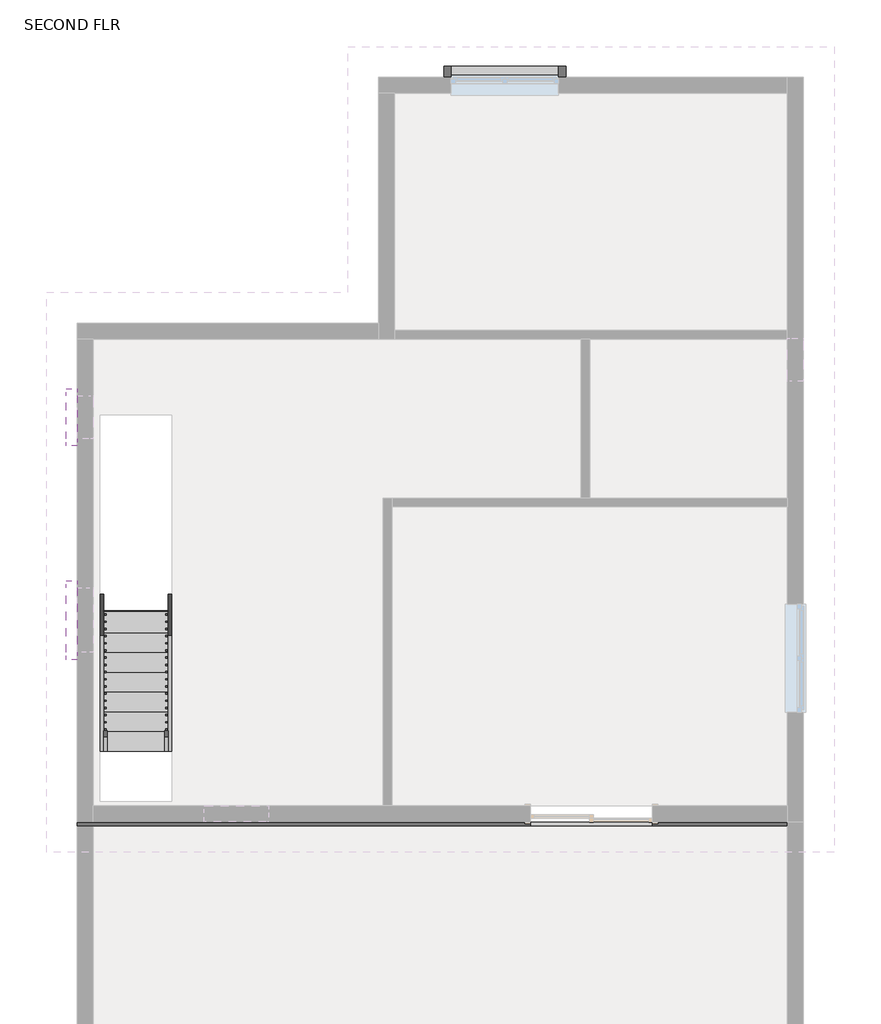
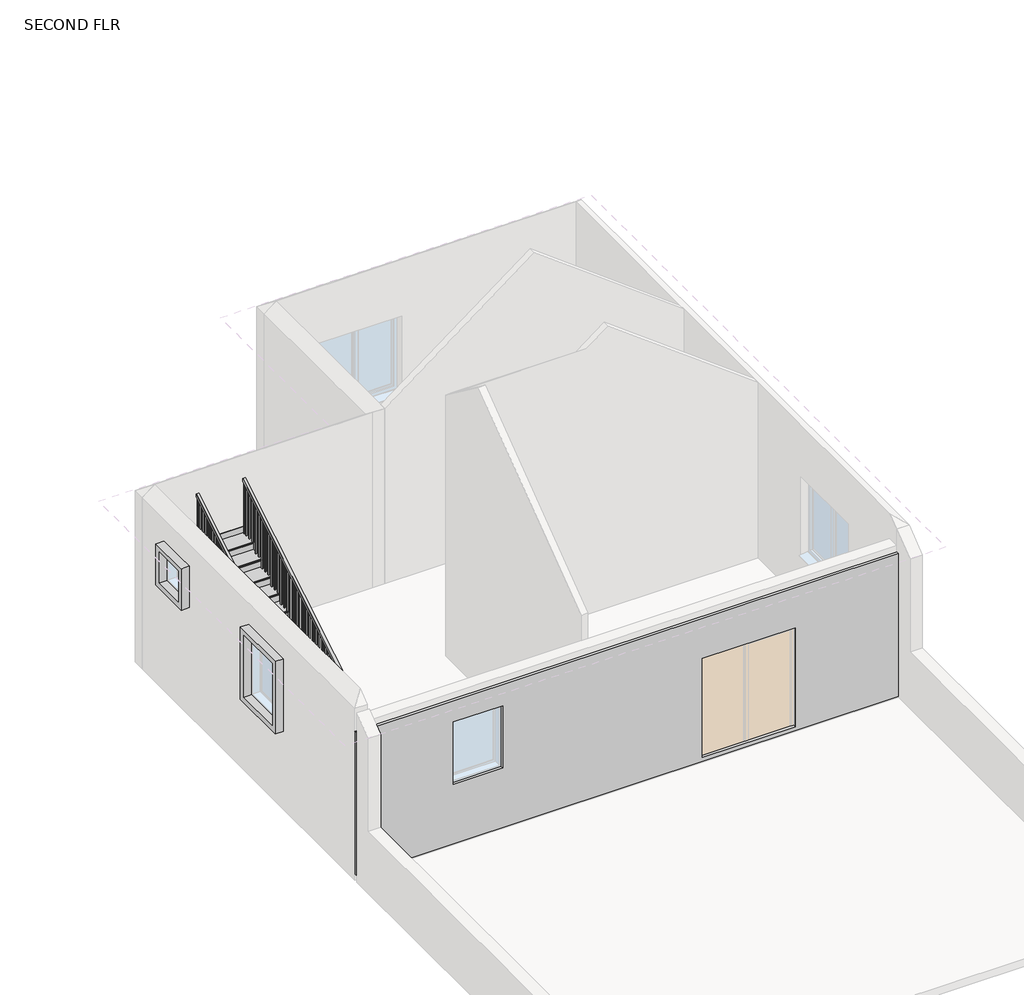
# One storey, part 2 of 2: 4 proxies, 2 members, 2 railings, 1 stair flight.
"""IFC4 building model written with IfcOpenShell, lengths in millimetres."""

from ifc_helpers import new_model, si_unit, frame, origin, place, context, project, spatial, polyline, outline, extrude, transform, mapped, element, save
from components import generic_models_10_generic_models_10_8dbd4941, generic_models_18_generic_models_18_bc45088a, generic_models_5_generic_models_5_2da6e60e, generic_models_9_generic_models_9_c35f1afa, stair_flight_ac41b8a3

model = new_model("IFC4")

# Units and contexts
model_context = context("Model", 3, world=origin())
ifc_project = project(units=[si_unit("LENGTHUNIT", "METRE", prefix="MILLI")], contexts=[model_context])

# Site, building, storey
site = spatial("IfcSite", under=ifc_project)
building = spatial("IfcBuilding", under=site)
storey = spatial("IfcBuildingStorey", under=building, Name="SECOND FLR", Elevation=6400.8)

# Proxies
placement = place(None, origin())
generic_models_10_generic_models_10_shape = generic_models_10_generic_models_10_8dbd4941(model_context)
element("IfcBuildingElementProxy", 1, Name="Generic Models 10 : Generic Models 10", ObjectType="Generic Models 10 : Generic Models 10", at=placement, inside=storey, context=model_context, shape_type="MappedRepresentation", body=[
    mapped(generic_models_10_generic_models_10_shape, transform((0.0, 0.0, 0.0), x_axis=(1.0, 0.0, 0.0), y_axis=(0.0, 1.0, 0.0), z_axis=(0.0, 0.0, 1.0))),
])
generic_models_18_generic_models_18_shape = generic_models_18_generic_models_18_bc45088a(model_context)
element("IfcBuildingElementProxy", 2, Name="Generic Models 18 : Generic Models 18", ObjectType="Generic Models 18 : Generic Models 18", at=placement, inside=storey, context=model_context, shape_type="MappedRepresentation", body=[
    mapped(generic_models_18_generic_models_18_shape, transform((0.0, 0.0, 0.0), x_axis=(1.0, 0.0, 0.0), y_axis=(0.0, 1.0, 0.0), z_axis=(0.0, 0.0, 1.0))),
])
generic_models_5_generic_models_5_shape = generic_models_5_generic_models_5_2da6e60e(model_context)
element("IfcBuildingElementProxy", 3, Name="Generic Models 5 : Generic Models 5", ObjectType="Generic Models 5 : Generic Models 5", at=placement, inside=storey, context=model_context, shape_type="MappedRepresentation", body=[
    mapped(generic_models_5_generic_models_5_shape, transform((0.0, 0.0, 0.0), x_axis=(1.0, 0.0, 0.0), y_axis=(0.0, 1.0, 0.0), z_axis=(0.0, 0.0, 1.0))),
])
generic_models_9_generic_models_9_shape = generic_models_9_generic_models_9_c35f1afa(model_context)
element("IfcBuildingElementProxy", 4, Name="Generic Models 9 : Generic Models 9", ObjectType="Generic Models 9 : Generic Models 9", at=placement, inside=storey, context=model_context, shape_type="MappedRepresentation", body=[
    mapped(generic_models_9_generic_models_9_shape, transform((0.0, 0.0, 0.0), x_axis=(1.0, 0.0, 0.0), y_axis=(0.0, 1.0, 0.0), z_axis=(0.0, 0.0, 1.0))),
])

# Members
element("IfcMember", 5, ObjectType="Stringer - 2\" Width", at=placement, inside=storey, context=model_context, shape_type="SweptSolid", body=[
    extrude(outline(polyline([(2731.9325341, 6400.8), (2731.9325341, 6612.914512), (7481.7325341, 9491.5811786), (7481.7325341, 9135.1724171), (2970.0180459, 6400.8), (2731.9325341, 6400.8)])), frame((-5772.3875748, 0.0, 0.0), z_axis=(1.0, 0.0, 0.0), x_axis=(0.0, 1.0, 0.0)), (0.0, 0.0, 1.0), 50.8),
])
element("IfcMember", 6, ObjectType="Stringer - 2\" Width", at=placement, inside=storey, context=model_context, shape_type="SweptSolid", body=[
    extrude(outline(polyline([(2731.9325341, 6400.8), (2731.9325341, 6612.914512), (7481.7325341, 9491.5811786), (7481.7325341, 9135.1724171), (2970.0180459, 6400.8), (2731.9325341, 6400.8)])), frame((-4807.1875748, 0.0, 0.0), z_axis=(1.0, 0.0, 0.0), x_axis=(0.0, 1.0, 0.0)), (0.0, 0.0, 1.0), 50.8),
])

# Railings
element("IfcRailing", 7, ObjectType="Handrail - Rectangular", at=placement, inside=storey, context=model_context, shape_type="SweptSolid", body=[
    extrude(outline(polyline([(2731.9325341, 7425.1318731), (2731.9325341, 7484.5333333), (7481.7325341, 10363.2), (7481.7325341, 10303.7985397), (2731.9325341, 7425.1318731)])), frame((-4857.9875748, 0.0, 0.0), z_axis=(1.0, 0.0, 0.0), x_axis=(0.0, 1.0, 0.0)), (0.0, 0.0, 1.0), 50.8),
    extrude(outline(polyline([(7396.0075341, 10251.8439943), (7415.0575341, 10263.3894488), (7415.0575341, 9279.4666667), (7396.0075341, 9279.4666667), (7396.0075341, 10251.8439943)])), frame((-4842.1125748, 0.0, 0.0), z_axis=(1.0, 0.0, 0.0), x_axis=(0.0, 1.0, 0.0)), (0.0, 0.0, 1.0), 19.05),
    extrude(outline(polyline([(7294.4075341, 10190.2682367), (7313.4575341, 10201.8136913), (7313.4575341, 9279.4666667), (7294.4075341, 9279.4666667), (7294.4075341, 10190.2682367)])), frame((-4842.1125748, 0.0, 0.0), z_axis=(1.0, 0.0, 0.0), x_axis=(0.0, 1.0, 0.0)), (0.0, 0.0, 1.0), 19.05),
    extrude(outline(polyline([(7192.8075341, 10128.6924791), (7211.8575341, 10140.2379337), (7211.8575341, 9279.4666667), (7192.8075341, 9279.4666667), (7192.8075341, 10128.6924791)])), frame((-4842.1125748, 0.0, 0.0), z_axis=(1.0, 0.0, 0.0), x_axis=(0.0, 1.0, 0.0)), (0.0, 0.0, 1.0), 19.05),
    extrude(outline(polyline([(7091.2075341, 10067.1167216), (7110.2575341, 10078.6621761), (7110.2575341, 9110.1333333), (7091.2075341, 9110.1333333), (7091.2075341, 10067.1167216)])), frame((-4842.1125748, 0.0, 0.0), z_axis=(1.0, 0.0, 0.0), x_axis=(0.0, 1.0, 0.0)), (0.0, 0.0, 1.0), 19.05),
    extrude(outline(polyline([(6989.6075341, 10005.540964), (7008.6575341, 10017.0864185), (7008.6575341, 9110.1333333), (6989.6075341, 9110.1333333), (6989.6075341, 10005.540964)])), frame((-4842.1125748, 0.0, 0.0), z_axis=(1.0, 0.0, 0.0), x_axis=(0.0, 1.0, 0.0)), (0.0, 0.0, 1.0), 19.05),
    extrude(outline(polyline([(6888.0075341, 9943.9652064), (6907.0575341, 9955.510661), (6907.0575341, 8940.8), (6888.0075341, 8940.8), (6888.0075341, 9943.9652064)])), frame((-4842.1125748, 0.0, 0.0), z_axis=(1.0, 0.0, 0.0), x_axis=(0.0, 1.0, 0.0)), (0.0, 0.0, 1.0), 19.05),
    extrude(outline(polyline([(6786.4075341, 9882.3894488), (6805.4575341, 9893.9349034), (6805.4575341, 8940.8), (6786.4075341, 8940.8), (6786.4075341, 9882.3894488)])), frame((-4842.1125748, 0.0, 0.0), z_axis=(1.0, 0.0, 0.0), x_axis=(0.0, 1.0, 0.0)), (0.0, 0.0, 1.0), 19.05),
    extrude(outline(polyline([(6684.8075341, 9820.8136913), (6703.8575341, 9832.3591458), (6703.8575341, 8940.8), (6684.8075341, 8940.8), (6684.8075341, 9820.8136913)])), frame((-4842.1125748, 0.0, 0.0), z_axis=(1.0, 0.0, 0.0), x_axis=(0.0, 1.0, 0.0)), (0.0, 0.0, 1.0), 19.05),
    extrude(outline(polyline([(6583.2075341, 9759.2379337), (6602.2575341, 9770.7833882), (6602.2575341, 8771.4666667), (6583.2075341, 8771.4666667), (6583.2075341, 9759.2379337)])), frame((-4842.1125748, 0.0, 0.0), z_axis=(1.0, 0.0, 0.0), x_axis=(0.0, 1.0, 0.0)), (0.0, 0.0, 1.0), 19.05),
    extrude(outline(polyline([(6481.6075341, 9697.6621761), (6500.6575341, 9709.2076307), (6500.6575341, 8771.4666667), (6481.6075341, 8771.4666667), (6481.6075341, 9697.6621761)])), frame((-4842.1125748, 0.0, 0.0), z_axis=(1.0, 0.0, 0.0), x_axis=(0.0, 1.0, 0.0)), (0.0, 0.0, 1.0), 19.05),
    extrude(outline(polyline([(6380.0075341, 9636.0864185), (6399.0575341, 9647.6318731), (6399.0575341, 8771.4666667), (6380.0075341, 8771.4666667), (6380.0075341, 9636.0864185)])), frame((-4842.1125748, 0.0, 0.0), z_axis=(1.0, 0.0, 0.0), x_axis=(0.0, 1.0, 0.0)), (0.0, 0.0, 1.0), 19.05),
    extrude(outline(polyline([(6278.4075341, 9574.510661), (6297.4575341, 9586.0561155), (6297.4575341, 8602.1333333), (6278.4075341, 8602.1333333), (6278.4075341, 9574.510661)])), frame((-4842.1125748, 0.0, 0.0), z_axis=(1.0, 0.0, 0.0), x_axis=(0.0, 1.0, 0.0)), (0.0, 0.0, 1.0), 19.05),
    extrude(outline(polyline([(6176.8075341, 9512.9349034), (6195.8575341, 9524.4803579), (6195.8575341, 8602.1333333), (6176.8075341, 8602.1333333), (6176.8075341, 9512.9349034)])), frame((-4842.1125748, 0.0, 0.0), z_axis=(1.0, 0.0, 0.0), x_axis=(0.0, 1.0, 0.0)), (0.0, 0.0, 1.0), 19.05),
    extrude(outline(polyline([(6075.2075341, 9451.3591458), (6094.2575341, 9462.9046004), (6094.2575341, 8602.1333333), (6075.2075341, 8602.1333333), (6075.2075341, 9451.3591458)])), frame((-4842.1125748, 0.0, 0.0), z_axis=(1.0, 0.0, 0.0), x_axis=(0.0, 1.0, 0.0)), (0.0, 0.0, 1.0), 19.05),
    extrude(outline(polyline([(5973.6075341, 9389.7833882), (5992.6575341, 9401.3288428), (5992.6575341, 8432.8), (5973.6075341, 8432.8), (5973.6075341, 9389.7833882)])), frame((-4842.1125748, 0.0, 0.0), z_axis=(1.0, 0.0, 0.0), x_axis=(0.0, 1.0, 0.0)), (0.0, 0.0, 1.0), 19.05),
    extrude(outline(polyline([(5872.0075341, 9328.2076307), (5891.0575341, 9339.7530852), (5891.0575341, 8432.8), (5872.0075341, 8432.8), (5872.0075341, 9328.2076307)])), frame((-4842.1125748, 0.0, 0.0), z_axis=(1.0, 0.0, 0.0), x_axis=(0.0, 1.0, 0.0)), (0.0, 0.0, 1.0), 19.05),
    extrude(outline(polyline([(5770.4075341, 9266.6318731), (5789.4575341, 9278.1773276), (5789.4575341, 8263.4666667), (5770.4075341, 8263.4666667), (5770.4075341, 9266.6318731)])), frame((-4842.1125748, 0.0, 0.0), z_axis=(1.0, 0.0, 0.0), x_axis=(0.0, 1.0, 0.0)), (0.0, 0.0, 1.0), 19.05),
    extrude(outline(polyline([(5668.8075341, 9205.0561155), (5687.8575341, 9216.6015701), (5687.8575341, 8263.4666667), (5668.8075341, 8263.4666667), (5668.8075341, 9205.0561155)])), frame((-4842.1125748, 0.0, 0.0), z_axis=(1.0, 0.0, 0.0), x_axis=(0.0, 1.0, 0.0)), (0.0, 0.0, 1.0), 19.05),
    extrude(outline(polyline([(5567.2075341, 9143.4803579), (5586.2575341, 9155.0258125), (5586.2575341, 8263.4666667), (5567.2075341, 8263.4666667), (5567.2075341, 9143.4803579)])), frame((-4842.1125748, 0.0, 0.0), z_axis=(1.0, 0.0, 0.0), x_axis=(0.0, 1.0, 0.0)), (0.0, 0.0, 1.0), 19.05),
    extrude(outline(polyline([(5465.6075341, 9081.9046004), (5484.6575341, 9093.4500549), (5484.6575341, 8094.1333333), (5465.6075341, 8094.1333333), (5465.6075341, 9081.9046004)])), frame((-4842.1125748, 0.0, 0.0), z_axis=(1.0, 0.0, 0.0), x_axis=(0.0, 1.0, 0.0)), (0.0, 0.0, 1.0), 19.05),
    extrude(outline(polyline([(5364.0075341, 9020.3288428), (5383.0575341, 9031.8742973), (5383.0575341, 8094.1333333), (5364.0075341, 8094.1333333), (5364.0075341, 9020.3288428)])), frame((-4842.1125748, 0.0, 0.0), z_axis=(1.0, 0.0, 0.0), x_axis=(0.0, 1.0, 0.0)), (0.0, 0.0, 1.0), 19.05),
    extrude(outline(polyline([(5262.4075341, 8958.7530852), (5281.4575341, 8970.2985397), (5281.4575341, 8094.1333333), (5262.4075341, 8094.1333333), (5262.4075341, 8958.7530852)])), frame((-4842.1125748, 0.0, 0.0), z_axis=(1.0, 0.0, 0.0), x_axis=(0.0, 1.0, 0.0)), (0.0, 0.0, 1.0), 19.05),
    extrude(outline(polyline([(5160.8075341, 8897.1773276), (5179.8575341, 8908.7227822), (5179.8575341, 7924.8), (5160.8075341, 7924.8), (5160.8075341, 8897.1773276)])), frame((-4842.1125748, 0.0, 0.0), z_axis=(1.0, 0.0, 0.0), x_axis=(0.0, 1.0, 0.0)), (0.0, 0.0, 1.0), 19.05),
    extrude(outline(polyline([(5059.2075341, 8835.6015701), (5078.2575341, 8847.1470246), (5078.2575341, 7924.8), (5059.2075341, 7924.8), (5059.2075341, 8835.6015701)])), frame((-4842.1125748, 0.0, 0.0), z_axis=(1.0, 0.0, 0.0), x_axis=(0.0, 1.0, 0.0)), (0.0, 0.0, 1.0), 19.05),
    extrude(outline(polyline([(4957.6075341, 8774.0258125), (4976.6575341, 8785.571267), (4976.6575341, 7924.8), (4957.6075341, 7924.8), (4957.6075341, 8774.0258125)])), frame((-4842.1125748, 0.0, 0.0), z_axis=(1.0, 0.0, 0.0), x_axis=(0.0, 1.0, 0.0)), (0.0, 0.0, 1.0), 19.05),
    extrude(outline(polyline([(4856.0075341, 8712.4500549), (4875.0575341, 8723.9955094), (4875.0575341, 7755.4666667), (4856.0075341, 7755.4666667), (4856.0075341, 8712.4500549)])), frame((-4842.1125748, 0.0, 0.0), z_axis=(1.0, 0.0, 0.0), x_axis=(0.0, 1.0, 0.0)), (0.0, 0.0, 1.0), 19.05),
    extrude(outline(polyline([(4754.4075341, 8650.8742973), (4773.4575341, 8662.4197519), (4773.4575341, 7755.4666667), (4754.4075341, 7755.4666667), (4754.4075341, 8650.8742973)])), frame((-4842.1125748, 0.0, 0.0), z_axis=(1.0, 0.0, 0.0), x_axis=(0.0, 1.0, 0.0)), (0.0, 0.0, 1.0), 19.05),
    extrude(outline(polyline([(4652.8075341, 8589.2985397), (4671.8575341, 8600.8439943), (4671.8575341, 7586.1333333), (4652.8075341, 7586.1333333), (4652.8075341, 8589.2985397)])), frame((-4842.1125748, 0.0, 0.0), z_axis=(1.0, 0.0, 0.0), x_axis=(0.0, 1.0, 0.0)), (0.0, 0.0, 1.0), 19.05),
    extrude(outline(polyline([(4551.2075341, 8527.7227822), (4570.2575341, 8539.2682367), (4570.2575341, 7586.1333333), (4551.2075341, 7586.1333333), (4551.2075341, 8527.7227822)])), frame((-4842.1125748, 0.0, 0.0), z_axis=(1.0, 0.0, 0.0), x_axis=(0.0, 1.0, 0.0)), (0.0, 0.0, 1.0), 19.05),
    extrude(outline(polyline([(4449.6075341, 8466.1470246), (4468.6575341, 8477.6924791), (4468.6575341, 7586.1333333), (4449.6075341, 7586.1333333), (4449.6075341, 8466.1470246)])), frame((-4842.1125748, 0.0, 0.0), z_axis=(1.0, 0.0, 0.0), x_axis=(0.0, 1.0, 0.0)), (0.0, 0.0, 1.0), 19.05),
    extrude(outline(polyline([(4348.0075341, 8404.571267), (4367.0575341, 8416.1167216), (4367.0575341, 7416.8), (4348.0075341, 7416.8), (4348.0075341, 8404.571267)])), frame((-4842.1125748, 0.0, 0.0), z_axis=(1.0, 0.0, 0.0), x_axis=(0.0, 1.0, 0.0)), (0.0, 0.0, 1.0), 19.05),
    extrude(outline(polyline([(4246.4075341, 8342.9955094), (4265.4575341, 8354.540964), (4265.4575341, 7416.8), (4246.4075341, 7416.8), (4246.4075341, 8342.9955094)])), frame((-4842.1125748, 0.0, 0.0), z_axis=(1.0, 0.0, 0.0), x_axis=(0.0, 1.0, 0.0)), (0.0, 0.0, 1.0), 19.05),
    extrude(outline(polyline([(4144.8075341, 8281.4197519), (4163.8575341, 8292.9652064), (4163.8575341, 7416.8), (4144.8075341, 7416.8), (4144.8075341, 8281.4197519)])), frame((-4842.1125748, 0.0, 0.0), z_axis=(1.0, 0.0, 0.0), x_axis=(0.0, 1.0, 0.0)), (0.0, 0.0, 1.0), 19.05),
    extrude(outline(polyline([(4043.2075341, 8219.8439943), (4062.2575341, 8231.3894488), (4062.2575341, 7247.4666667), (4043.2075341, 7247.4666667), (4043.2075341, 8219.8439943)])), frame((-4842.1125748, 0.0, 0.0), z_axis=(1.0, 0.0, 0.0), x_axis=(0.0, 1.0, 0.0)), (0.0, 0.0, 1.0), 19.05),
    extrude(outline(polyline([(3941.6075341, 8158.2682367), (3960.6575341, 8169.8136913), (3960.6575341, 7247.4666667), (3941.6075341, 7247.4666667), (3941.6075341, 8158.2682367)])), frame((-4842.1125748, 0.0, 0.0), z_axis=(1.0, 0.0, 0.0), x_axis=(0.0, 1.0, 0.0)), (0.0, 0.0, 1.0), 19.05),
    extrude(outline(polyline([(3840.0075341, 8096.6924791), (3859.0575341, 8108.2379337), (3859.0575341, 7247.4666667), (3840.0075341, 7247.4666667), (3840.0075341, 8096.6924791)])), frame((-4842.1125748, 0.0, 0.0), z_axis=(1.0, 0.0, 0.0), x_axis=(0.0, 1.0, 0.0)), (0.0, 0.0, 1.0), 19.05),
    extrude(outline(polyline([(3738.4075341, 8035.1167216), (3757.4575341, 8046.6621761), (3757.4575341, 7078.1333333), (3738.4075341, 7078.1333333), (3738.4075341, 8035.1167216)])), frame((-4842.1125748, 0.0, 0.0), z_axis=(1.0, 0.0, 0.0), x_axis=(0.0, 1.0, 0.0)), (0.0, 0.0, 1.0), 19.05),
    extrude(outline(polyline([(3636.8075341, 7973.540964), (3655.8575341, 7985.0864185), (3655.8575341, 7078.1333333), (3636.8075341, 7078.1333333), (3636.8075341, 7973.540964)])), frame((-4842.1125748, 0.0, 0.0), z_axis=(1.0, 0.0, 0.0), x_axis=(0.0, 1.0, 0.0)), (0.0, 0.0, 1.0), 19.05),
    extrude(outline(polyline([(3535.2075341, 7911.9652064), (3554.2575341, 7923.510661), (3554.2575341, 6908.8), (3535.2075341, 6908.8), (3535.2075341, 7911.9652064)])), frame((-4842.1125748, 0.0, 0.0), z_axis=(1.0, 0.0, 0.0), x_axis=(0.0, 1.0, 0.0)), (0.0, 0.0, 1.0), 19.05),
    extrude(outline(polyline([(3433.6075341, 7850.3894488), (3452.6575341, 7861.9349034), (3452.6575341, 6908.8), (3433.6075341, 6908.8), (3433.6075341, 7850.3894488)])), frame((-4842.1125748, 0.0, 0.0), z_axis=(1.0, 0.0, 0.0), x_axis=(0.0, 1.0, 0.0)), (0.0, 0.0, 1.0), 19.05),
    extrude(outline(polyline([(3332.0075341, 7788.8136913), (3351.0575341, 7800.3591458), (3351.0575341, 6908.8), (3332.0075341, 6908.8), (3332.0075341, 7788.8136913)])), frame((-4842.1125748, 0.0, 0.0), z_axis=(1.0, 0.0, 0.0), x_axis=(0.0, 1.0, 0.0)), (0.0, 0.0, 1.0), 19.05),
    extrude(outline(polyline([(3230.4075341, 7727.2379337), (3249.4575341, 7738.7833882), (3249.4575341, 6739.4666667), (3230.4075341, 6739.4666667), (3230.4075341, 7727.2379337)])), frame((-4842.1125748, 0.0, 0.0), z_axis=(1.0, 0.0, 0.0), x_axis=(0.0, 1.0, 0.0)), (0.0, 0.0, 1.0), 19.05),
    extrude(outline(polyline([(3128.8075341, 7665.6621761), (3147.8575341, 7677.2076307), (3147.8575341, 6739.4666667), (3128.8075341, 6739.4666667), (3128.8075341, 7665.6621761)])), frame((-4842.1125748, 0.0, 0.0), z_axis=(1.0, 0.0, 0.0), x_axis=(0.0, 1.0, 0.0)), (0.0, 0.0, 1.0), 19.05),
    extrude(outline(polyline([(3027.2075341, 7604.0864185), (3046.2575341, 7615.6318731), (3046.2575341, 6739.4666667), (3027.2075341, 6739.4666667), (3027.2075341, 7604.0864185)])), frame((-4842.1125748, 0.0, 0.0), z_axis=(1.0, 0.0, 0.0), x_axis=(0.0, 1.0, 0.0)), (0.0, 0.0, 1.0), 19.05),
    extrude(outline(polyline([(2925.6075341, 7542.510661), (2944.6575341, 7554.0561155), (2944.6575341, 6570.1333333), (2925.6075341, 6570.1333333), (2925.6075341, 7542.510661)])), frame((-4842.1125748, 0.0, 0.0), z_axis=(1.0, 0.0, 0.0), x_axis=(0.0, 1.0, 0.0)), (0.0, 0.0, 1.0), 19.05),
    extrude(outline(polyline([(2824.0075341, 7480.9349034), (2843.0575341, 7492.4803579), (2843.0575341, 6570.1333333), (2824.0075341, 6570.1333333), (2824.0075341, 7480.9349034)])), frame((-4842.1125748, 0.0, 0.0), z_axis=(1.0, 0.0, 0.0), x_axis=(0.0, 1.0, 0.0)), (0.0, 0.0, 1.0), 19.05),
    extrude(outline(polyline([(7462.6825341, 10292.2530852), (7481.7325341, 10303.7985397), (7481.7325341, 9279.4666667), (7462.6825341, 9279.4666667), (7462.6825341, 10292.2530852)])), frame((-4842.1125748, 0.0, 0.0), z_axis=(1.0, 0.0, 0.0), x_axis=(0.0, 1.0, 0.0)), (0.0, 0.0, 1.0), 19.05),
    extrude(outline(polyline([(2731.9325341, 7425.1318731), (2750.9825341, 7436.6773276), (2750.9825341, 6570.1333333), (2731.9325341, 6570.1333333), (2731.9325341, 7425.1318731)])), frame((-4842.1125748, 0.0, 0.0), z_axis=(1.0, 0.0, 0.0), x_axis=(0.0, 1.0, 0.0)), (0.0, 0.0, 1.0), 19.05),
])
element("IfcRailing", 8, ObjectType="Handrail - Rectangular", at=placement, inside=storey, context=model_context, shape_type="SweptSolid", body=[
    extrude(outline(polyline([(2731.9325341, 7425.1318731), (2731.9325341, 7484.5333333), (7481.7325341, 10363.2), (7481.7325341, 10303.7985397), (2731.9325341, 7425.1318731)])), frame((-5721.5875748, 0.0, 0.0), z_axis=(1.0, 0.0, 0.0), x_axis=(0.0, 1.0, 0.0)), (0.0, 0.0, 1.0), 50.8),
    extrude(outline(polyline([(7415.0575341, 10263.3894488), (7415.0575341, 9279.4666667), (7396.0075341, 9279.4666667), (7396.0075341, 10251.8439943), (7415.0575341, 10263.3894488)])), frame((-5705.7125748, 0.0, 0.0), z_axis=(1.0, 0.0, 0.0), x_axis=(0.0, 1.0, 0.0)), (0.0, 0.0, 1.0), 19.05),
    extrude(outline(polyline([(7313.4575341, 10201.8136913), (7313.4575341, 9279.4666667), (7294.4075341, 9279.4666667), (7294.4075341, 10190.2682367), (7313.4575341, 10201.8136913)])), frame((-5705.7125748, 0.0, 0.0), z_axis=(1.0, 0.0, 0.0), x_axis=(0.0, 1.0, 0.0)), (0.0, 0.0, 1.0), 19.05),
    extrude(outline(polyline([(7211.8575341, 10140.2379337), (7211.8575341, 9279.4666667), (7192.8075341, 9279.4666667), (7192.8075341, 10128.6924791), (7211.8575341, 10140.2379337)])), frame((-5705.7125748, 0.0, 0.0), z_axis=(1.0, 0.0, 0.0), x_axis=(0.0, 1.0, 0.0)), (0.0, 0.0, 1.0), 19.05),
    extrude(outline(polyline([(7110.2575341, 10078.6621761), (7110.2575341, 9110.1333333), (7091.2075341, 9110.1333333), (7091.2075341, 10067.1167216), (7110.2575341, 10078.6621761)])), frame((-5705.7125748, 0.0, 0.0), z_axis=(1.0, 0.0, 0.0), x_axis=(0.0, 1.0, 0.0)), (0.0, 0.0, 1.0), 19.05),
    extrude(outline(polyline([(7008.6575341, 10017.0864185), (7008.6575341, 9110.1333333), (6989.6075341, 9110.1333333), (6989.6075341, 10005.540964), (7008.6575341, 10017.0864185)])), frame((-5705.7125748, 0.0, 0.0), z_axis=(1.0, 0.0, 0.0), x_axis=(0.0, 1.0, 0.0)), (0.0, 0.0, 1.0), 19.05),
    extrude(outline(polyline([(6907.0575341, 9955.510661), (6907.0575341, 8940.8), (6888.0075341, 8940.8), (6888.0075341, 9943.9652064), (6907.0575341, 9955.510661)])), frame((-5705.7125748, 0.0, 0.0), z_axis=(1.0, 0.0, 0.0), x_axis=(0.0, 1.0, 0.0)), (0.0, 0.0, 1.0), 19.05),
    extrude(outline(polyline([(6805.4575341, 9893.9349034), (6805.4575341, 8940.8), (6786.4075341, 8940.8), (6786.4075341, 9882.3894488), (6805.4575341, 9893.9349034)])), frame((-5705.7125748, 0.0, 0.0), z_axis=(1.0, 0.0, 0.0), x_axis=(0.0, 1.0, 0.0)), (0.0, 0.0, 1.0), 19.05),
    extrude(outline(polyline([(6703.8575341, 9832.3591458), (6703.8575341, 8940.8), (6684.8075341, 8940.8), (6684.8075341, 9820.8136913), (6703.8575341, 9832.3591458)])), frame((-5705.7125748, 0.0, 0.0), z_axis=(1.0, 0.0, 0.0), x_axis=(0.0, 1.0, 0.0)), (0.0, 0.0, 1.0), 19.05),
    extrude(outline(polyline([(6602.2575341, 9770.7833882), (6602.2575341, 8771.4666667), (6583.2075341, 8771.4666667), (6583.2075341, 9759.2379337), (6602.2575341, 9770.7833882)])), frame((-5705.7125748, 0.0, 0.0), z_axis=(1.0, 0.0, 0.0), x_axis=(0.0, 1.0, 0.0)), (0.0, 0.0, 1.0), 19.05),
    extrude(outline(polyline([(6500.6575341, 9709.2076307), (6500.6575341, 8771.4666667), (6481.6075341, 8771.4666667), (6481.6075341, 9697.6621761), (6500.6575341, 9709.2076307)])), frame((-5705.7125748, 0.0, 0.0), z_axis=(1.0, 0.0, 0.0), x_axis=(0.0, 1.0, 0.0)), (0.0, 0.0, 1.0), 19.05),
    extrude(outline(polyline([(6399.0575341, 9647.6318731), (6399.0575341, 8771.4666667), (6380.0075341, 8771.4666667), (6380.0075341, 9636.0864185), (6399.0575341, 9647.6318731)])), frame((-5705.7125748, 0.0, 0.0), z_axis=(1.0, 0.0, 0.0), x_axis=(0.0, 1.0, 0.0)), (0.0, 0.0, 1.0), 19.05),
    extrude(outline(polyline([(6297.4575341, 9586.0561155), (6297.4575341, 8602.1333333), (6278.4075341, 8602.1333333), (6278.4075341, 9574.510661), (6297.4575341, 9586.0561155)])), frame((-5705.7125748, 0.0, 0.0), z_axis=(1.0, 0.0, 0.0), x_axis=(0.0, 1.0, 0.0)), (0.0, 0.0, 1.0), 19.05),
    extrude(outline(polyline([(6195.8575341, 9524.4803579), (6195.8575341, 8602.1333333), (6176.8075341, 8602.1333333), (6176.8075341, 9512.9349034), (6195.8575341, 9524.4803579)])), frame((-5705.7125748, 0.0, 0.0), z_axis=(1.0, 0.0, 0.0), x_axis=(0.0, 1.0, 0.0)), (0.0, 0.0, 1.0), 19.05),
    extrude(outline(polyline([(6094.2575341, 9462.9046004), (6094.2575341, 8602.1333333), (6075.2075341, 8602.1333333), (6075.2075341, 9451.3591458), (6094.2575341, 9462.9046004)])), frame((-5705.7125748, 0.0, 0.0), z_axis=(1.0, 0.0, 0.0), x_axis=(0.0, 1.0, 0.0)), (0.0, 0.0, 1.0), 19.05),
    extrude(outline(polyline([(5992.6575341, 9401.3288428), (5992.6575341, 8432.8), (5973.6075341, 8432.8), (5973.6075341, 9389.7833882), (5992.6575341, 9401.3288428)])), frame((-5705.7125748, 0.0, 0.0), z_axis=(1.0, 0.0, 0.0), x_axis=(0.0, 1.0, 0.0)), (0.0, 0.0, 1.0), 19.05),
    extrude(outline(polyline([(5891.0575341, 9339.7530852), (5891.0575341, 8432.8), (5872.0075341, 8432.8), (5872.0075341, 9328.2076307), (5891.0575341, 9339.7530852)])), frame((-5705.7125748, 0.0, 0.0), z_axis=(1.0, 0.0, 0.0), x_axis=(0.0, 1.0, 0.0)), (0.0, 0.0, 1.0), 19.05),
    extrude(outline(polyline([(5789.4575341, 9278.1773276), (5789.4575341, 8263.4666667), (5770.4075341, 8263.4666667), (5770.4075341, 9266.6318731), (5789.4575341, 9278.1773276)])), frame((-5705.7125748, 0.0, 0.0), z_axis=(1.0, 0.0, 0.0), x_axis=(0.0, 1.0, 0.0)), (0.0, 0.0, 1.0), 19.05),
    extrude(outline(polyline([(5687.8575341, 9216.6015701), (5687.8575341, 8263.4666667), (5668.8075341, 8263.4666667), (5668.8075341, 9205.0561155), (5687.8575341, 9216.6015701)])), frame((-5705.7125748, 0.0, 0.0), z_axis=(1.0, 0.0, 0.0), x_axis=(0.0, 1.0, 0.0)), (0.0, 0.0, 1.0), 19.05),
    extrude(outline(polyline([(5586.2575341, 9155.0258125), (5586.2575341, 8263.4666667), (5567.2075341, 8263.4666667), (5567.2075341, 9143.4803579), (5586.2575341, 9155.0258125)])), frame((-5705.7125748, 0.0, 0.0), z_axis=(1.0, 0.0, 0.0), x_axis=(0.0, 1.0, 0.0)), (0.0, 0.0, 1.0), 19.05),
    extrude(outline(polyline([(5484.6575341, 9093.4500549), (5484.6575341, 8094.1333333), (5465.6075341, 8094.1333333), (5465.6075341, 9081.9046004), (5484.6575341, 9093.4500549)])), frame((-5705.7125748, 0.0, 0.0), z_axis=(1.0, 0.0, 0.0), x_axis=(0.0, 1.0, 0.0)), (0.0, 0.0, 1.0), 19.05),
    extrude(outline(polyline([(5383.0575341, 9031.8742973), (5383.0575341, 8094.1333333), (5364.0075341, 8094.1333333), (5364.0075341, 9020.3288428), (5383.0575341, 9031.8742973)])), frame((-5705.7125748, 0.0, 0.0), z_axis=(1.0, 0.0, 0.0), x_axis=(0.0, 1.0, 0.0)), (0.0, 0.0, 1.0), 19.05),
    extrude(outline(polyline([(5281.4575341, 8970.2985397), (5281.4575341, 8094.1333333), (5262.4075341, 8094.1333333), (5262.4075341, 8958.7530852), (5281.4575341, 8970.2985397)])), frame((-5705.7125748, 0.0, 0.0), z_axis=(1.0, 0.0, 0.0), x_axis=(0.0, 1.0, 0.0)), (0.0, 0.0, 1.0), 19.05),
    extrude(outline(polyline([(5179.8575341, 8908.7227822), (5179.8575341, 7924.8), (5160.8075341, 7924.8), (5160.8075341, 8897.1773276), (5179.8575341, 8908.7227822)])), frame((-5705.7125748, 0.0, 0.0), z_axis=(1.0, 0.0, 0.0), x_axis=(0.0, 1.0, 0.0)), (0.0, 0.0, 1.0), 19.05),
    extrude(outline(polyline([(5078.2575341, 8847.1470246), (5078.2575341, 7924.8), (5059.2075341, 7924.8), (5059.2075341, 8835.6015701), (5078.2575341, 8847.1470246)])), frame((-5705.7125748, 0.0, 0.0), z_axis=(1.0, 0.0, 0.0), x_axis=(0.0, 1.0, 0.0)), (0.0, 0.0, 1.0), 19.05),
    extrude(outline(polyline([(4976.6575341, 8785.571267), (4976.6575341, 7924.8), (4957.6075341, 7924.8), (4957.6075341, 8774.0258125), (4976.6575341, 8785.571267)])), frame((-5705.7125748, 0.0, 0.0), z_axis=(1.0, 0.0, 0.0), x_axis=(0.0, 1.0, 0.0)), (0.0, 0.0, 1.0), 19.05),
    extrude(outline(polyline([(4875.0575341, 8723.9955094), (4875.0575341, 7755.4666667), (4856.0075341, 7755.4666667), (4856.0075341, 8712.4500549), (4875.0575341, 8723.9955094)])), frame((-5705.7125748, 0.0, 0.0), z_axis=(1.0, 0.0, 0.0), x_axis=(0.0, 1.0, 0.0)), (0.0, 0.0, 1.0), 19.05),
    extrude(outline(polyline([(4773.4575341, 8662.4197519), (4773.4575341, 7755.4666667), (4754.4075341, 7755.4666667), (4754.4075341, 8650.8742973), (4773.4575341, 8662.4197519)])), frame((-5705.7125748, 0.0, 0.0), z_axis=(1.0, 0.0, 0.0), x_axis=(0.0, 1.0, 0.0)), (0.0, 0.0, 1.0), 19.05),
    extrude(outline(polyline([(4671.8575341, 8600.8439943), (4671.8575341, 7586.1333333), (4652.8075341, 7586.1333333), (4652.8075341, 8589.2985397), (4671.8575341, 8600.8439943)])), frame((-5705.7125748, 0.0, 0.0), z_axis=(1.0, 0.0, 0.0), x_axis=(0.0, 1.0, 0.0)), (0.0, 0.0, 1.0), 19.05),
    extrude(outline(polyline([(4570.2575341, 8539.2682367), (4570.2575341, 7586.1333333), (4551.2075341, 7586.1333333), (4551.2075341, 8527.7227822), (4570.2575341, 8539.2682367)])), frame((-5705.7125748, 0.0, 0.0), z_axis=(1.0, 0.0, 0.0), x_axis=(0.0, 1.0, 0.0)), (0.0, 0.0, 1.0), 19.05),
    extrude(outline(polyline([(4468.6575341, 8477.6924791), (4468.6575341, 7586.1333333), (4449.6075341, 7586.1333333), (4449.6075341, 8466.1470246), (4468.6575341, 8477.6924791)])), frame((-5705.7125748, 0.0, 0.0), z_axis=(1.0, 0.0, 0.0), x_axis=(0.0, 1.0, 0.0)), (0.0, 0.0, 1.0), 19.05),
    extrude(outline(polyline([(4367.0575341, 8416.1167216), (4367.0575341, 7416.8), (4348.0075341, 7416.8), (4348.0075341, 8404.571267), (4367.0575341, 8416.1167216)])), frame((-5705.7125748, 0.0, 0.0), z_axis=(1.0, 0.0, 0.0), x_axis=(0.0, 1.0, 0.0)), (0.0, 0.0, 1.0), 19.05),
    extrude(outline(polyline([(4265.4575341, 8354.540964), (4265.4575341, 7416.8), (4246.4075341, 7416.8), (4246.4075341, 8342.9955094), (4265.4575341, 8354.540964)])), frame((-5705.7125748, 0.0, 0.0), z_axis=(1.0, 0.0, 0.0), x_axis=(0.0, 1.0, 0.0)), (0.0, 0.0, 1.0), 19.05),
    extrude(outline(polyline([(4163.8575341, 8292.9652064), (4163.8575341, 7416.8), (4144.8075341, 7416.8), (4144.8075341, 8281.4197519), (4163.8575341, 8292.9652064)])), frame((-5705.7125748, 0.0, 0.0), z_axis=(1.0, 0.0, 0.0), x_axis=(0.0, 1.0, 0.0)), (0.0, 0.0, 1.0), 19.05),
    extrude(outline(polyline([(4062.2575341, 8231.3894488), (4062.2575341, 7247.4666667), (4043.2075341, 7247.4666667), (4043.2075341, 8219.8439943), (4062.2575341, 8231.3894488)])), frame((-5705.7125748, 0.0, 0.0), z_axis=(1.0, 0.0, 0.0), x_axis=(0.0, 1.0, 0.0)), (0.0, 0.0, 1.0), 19.05),
    extrude(outline(polyline([(3960.6575341, 8169.8136913), (3960.6575341, 7247.4666667), (3941.6075341, 7247.4666667), (3941.6075341, 8158.2682367), (3960.6575341, 8169.8136913)])), frame((-5705.7125748, 0.0, 0.0), z_axis=(1.0, 0.0, 0.0), x_axis=(0.0, 1.0, 0.0)), (0.0, 0.0, 1.0), 19.05),
    extrude(outline(polyline([(3859.0575341, 8108.2379337), (3859.0575341, 7247.4666667), (3840.0075341, 7247.4666667), (3840.0075341, 8096.6924791), (3859.0575341, 8108.2379337)])), frame((-5705.7125748, 0.0, 0.0), z_axis=(1.0, 0.0, 0.0), x_axis=(0.0, 1.0, 0.0)), (0.0, 0.0, 1.0), 19.05),
    extrude(outline(polyline([(3757.4575341, 8046.6621761), (3757.4575341, 7078.1333333), (3738.4075341, 7078.1333333), (3738.4075341, 8035.1167216), (3757.4575341, 8046.6621761)])), frame((-5705.7125748, 0.0, 0.0), z_axis=(1.0, 0.0, 0.0), x_axis=(0.0, 1.0, 0.0)), (0.0, 0.0, 1.0), 19.05),
    extrude(outline(polyline([(3655.8575341, 7985.0864185), (3655.8575341, 7078.1333333), (3636.8075341, 7078.1333333), (3636.8075341, 7973.540964), (3655.8575341, 7985.0864185)])), frame((-5705.7125748, 0.0, 0.0), z_axis=(1.0, 0.0, 0.0), x_axis=(0.0, 1.0, 0.0)), (0.0, 0.0, 1.0), 19.05),
    extrude(outline(polyline([(3554.2575341, 7923.510661), (3554.2575341, 6908.8), (3535.2075341, 6908.8), (3535.2075341, 7911.9652064), (3554.2575341, 7923.510661)])), frame((-5705.7125748, 0.0, 0.0), z_axis=(1.0, 0.0, 0.0), x_axis=(0.0, 1.0, 0.0)), (0.0, 0.0, 1.0), 19.05),
    extrude(outline(polyline([(3452.6575341, 7861.9349034), (3452.6575341, 6908.8), (3433.6075341, 6908.8), (3433.6075341, 7850.3894488), (3452.6575341, 7861.9349034)])), frame((-5705.7125748, 0.0, 0.0), z_axis=(1.0, 0.0, 0.0), x_axis=(0.0, 1.0, 0.0)), (0.0, 0.0, 1.0), 19.05),
    extrude(outline(polyline([(3351.0575341, 7800.3591458), (3351.0575341, 6908.8), (3332.0075341, 6908.8), (3332.0075341, 7788.8136913), (3351.0575341, 7800.3591458)])), frame((-5705.7125748, 0.0, 0.0), z_axis=(1.0, 0.0, 0.0), x_axis=(0.0, 1.0, 0.0)), (0.0, 0.0, 1.0), 19.05),
    extrude(outline(polyline([(3249.4575341, 7738.7833882), (3249.4575341, 6739.4666667), (3230.4075341, 6739.4666667), (3230.4075341, 7727.2379337), (3249.4575341, 7738.7833882)])), frame((-5705.7125748, 0.0, 0.0), z_axis=(1.0, 0.0, 0.0), x_axis=(0.0, 1.0, 0.0)), (0.0, 0.0, 1.0), 19.05),
    extrude(outline(polyline([(3147.8575341, 7677.2076307), (3147.8575341, 6739.4666667), (3128.8075341, 6739.4666667), (3128.8075341, 7665.6621761), (3147.8575341, 7677.2076307)])), frame((-5705.7125748, 0.0, 0.0), z_axis=(1.0, 0.0, 0.0), x_axis=(0.0, 1.0, 0.0)), (0.0, 0.0, 1.0), 19.05),
    extrude(outline(polyline([(3046.2575341, 7615.6318731), (3046.2575341, 6739.4666667), (3027.2075341, 6739.4666667), (3027.2075341, 7604.0864185), (3046.2575341, 7615.6318731)])), frame((-5705.7125748, 0.0, 0.0), z_axis=(1.0, 0.0, 0.0), x_axis=(0.0, 1.0, 0.0)), (0.0, 0.0, 1.0), 19.05),
    extrude(outline(polyline([(2944.6575341, 7554.0561155), (2944.6575341, 6570.1333333), (2925.6075341, 6570.1333333), (2925.6075341, 7542.510661), (2944.6575341, 7554.0561155)])), frame((-5705.7125748, 0.0, 0.0), z_axis=(1.0, 0.0, 0.0), x_axis=(0.0, 1.0, 0.0)), (0.0, 0.0, 1.0), 19.05),
    extrude(outline(polyline([(2843.0575341, 7492.4803579), (2843.0575341, 6570.1333333), (2824.0075341, 6570.1333333), (2824.0075341, 7480.9349034), (2843.0575341, 7492.4803579)])), frame((-5705.7125748, 0.0, 0.0), z_axis=(1.0, 0.0, 0.0), x_axis=(0.0, 1.0, 0.0)), (0.0, 0.0, 1.0), 19.05),
    extrude(outline(polyline([(7481.7325341, 10303.7985397), (7481.7325341, 9279.4666667), (7462.6825341, 9279.4666667), (7462.6825341, 10292.2530852), (7481.7325341, 10303.7985397)])), frame((-5705.7125748, 0.0, 0.0), z_axis=(1.0, 0.0, 0.0), x_axis=(0.0, 1.0, 0.0)), (0.0, 0.0, 1.0), 19.05),
    extrude(outline(polyline([(2750.9825341, 7436.6773276), (2750.9825341, 6570.1333333), (2731.9325341, 6570.1333333), (2731.9325341, 7425.1318731), (2750.9825341, 7436.6773276)])), frame((-5705.7125748, 0.0, 0.0), z_axis=(1.0, 0.0, 0.0), x_axis=(0.0, 1.0, 0.0)), (0.0, 0.0, 1.0), 19.05),
])

# Stair flight
stair_flight_shape = stair_flight_ac41b8a3(model_context)
element("IfcStairFlight", 9, ObjectType="2\" Tread 1\" Nosing 1/4\" Riser", at=placement, inside=storey, context=model_context, shape_type="MappedRepresentation", body=[
    mapped(stair_flight_shape, transform((0.0, 0.0, 0.0), x_axis=(1.0, 0.0, 0.0), y_axis=(0.0, 1.0, 0.0), z_axis=(0.0, 0.0, 1.0))),
])

save(model, "model.ifc")

# Revit data of these elements
# Type "Handrail - Rectangular"
#   Assembly Code = "C2010400"
#   built-in parameter 1008612 = 0.0416667 (stored number, unit not read)
#   built-in parameter 1008611 = 0.0416667 (stored number, unit not read)
#   built-in parameter 1008609 = 0.333333 (stored number, unit not read)
#   built-in parameter 1008604 = 0.166667 (stored number, unit not read)
#   built-in parameter 1008603 = 0.166667 (stored number, unit not read)
#   Railing Height = 3' - 0"
#   built-in parameter 1008630 = 2
#   built-in parameter 1008610 = 2
#   built-in parameter 1008618 = Baluster - Square : 3/4"
# Element 1 (IfcBuildingElementProxy, "Generic Models 10 : Generic Models 10")
#   Phase Created = New Construction
#   Materials on its faces: "chocolate brown"
# Element 2 (IfcBuildingElementProxy, "Generic Models 18 : Generic Models 18")
#   Phase Created = New Construction
#   Materials on its faces: "chocolate brown"
# Element 3 (IfcBuildingElementProxy, "Generic Models 5 : Generic Models 5")
#   Phase Created = New Construction
# Element 4 (IfcBuildingElementProxy, "Generic Models 9 : Generic Models 9")
#   Phase Created = New Construction
#   Materials on its faces: "chocolate brown"
# Elements 5, 6 (IfcMember, "Stringer - 2\" Width")
#   Phase Created = New Construction
# Elements 7, 8 (IfcRailing, "Handrail - Rectangular")
#   Phase Created = New Construction
# Element 9 (IfcStairFlight, "2\" Tread 1\" Nosing 1/4\" Riser")
#   Phase Created = New Construction
# Materials
#   "chocolate brown": class "Generic", colour RGB 120 120 120, transparency 0, Cost = 0
